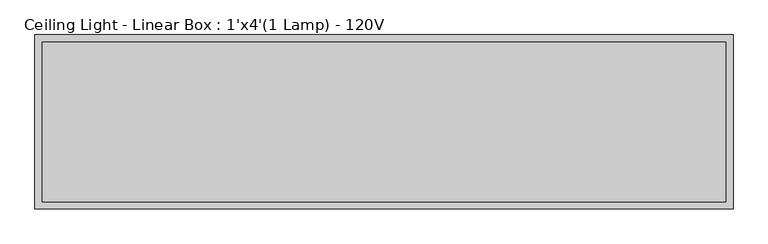
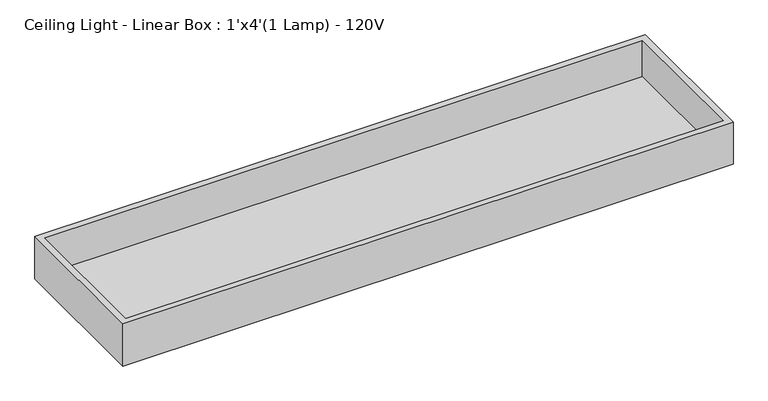
"""IFC4 building model written with IfcOpenShell, lengths in millimetres: light fixture geometry, Ceiling Light - Linear Box : 1'x4'(1 Lamp) - 120V."""

from ifc_helpers import new_model, si_unit, frame, origin, place, context, project, spatial, polyline, outline, extrude, source, transform, mapped, element, save


def ceiling_light_linear_box_1_x4_1_lamp_120v_8873ebfc(model_context):
    return source(origin(), model_context, "Body", "SweptSolid", [
        extrude(outline(polyline([(596.9, 139.7), (596.9, -139.7), (-596.9, -139.7), (-596.9, 139.7), (596.9, 139.7)])), frame((0.0, 0.0, 2355.85), z_axis=(0.0, 0.0, 1.0), x_axis=(1.0, 0.0, 0.0)), (0.0, 0.0, 1.0), 6.35),
        extrude(outline(polyline([(609.6, 152.4), (609.6, -152.4), (-609.6, -152.4), (-609.6, 152.4), (609.6, 152.4)]), holes=[polyline([(596.9, 139.7), (-596.9, 139.7), (-596.9, -139.7), (596.9, -139.7), (596.9, 139.7)])]), frame((0.0, 0.0, 2349.5), z_axis=(0.0, 0.0, 1.0), x_axis=(1.0, 0.0, 0.0)), (0.0, 0.0, 1.0), 88.9),
    ])


if __name__ == "__main__":
    model = new_model("IFC4")
    model_context = context("Model", 3, world=origin())
    ifc_project = project(units=[si_unit("LENGTHUNIT", "METRE", prefix="MILLI")], contexts=[model_context])
    site = spatial("IfcSite", under=ifc_project)
    building = spatial("IfcBuilding", under=site)
    placement = place(None, origin())
    ceiling_light_linear_box_1_x4_1_lamp_120v_shape = ceiling_light_linear_box_1_x4_1_lamp_120v_8873ebfc(model_context)
    element("IfcLightFixture", 1, ObjectType="Ceiling Light - Linear Box : 1'x4'(1 Lamp) - 120V", at=placement, inside=building, context=model_context, shape_type="MappedRepresentation", body=[
        mapped(ceiling_light_linear_box_1_x4_1_lamp_120v_shape, transform((0.0, 0.0, 0.0), x_axis=(1.0, 0.0, 0.0), y_axis=(0.0, 1.0, 0.0), z_axis=(0.0, 0.0, 1.0))),
    ])
    save(model, "model.ifc")

# Revit data of these elements
# Type "Ceiling Light - Linear Box : 1'x4'(1 Lamp) - 120V"
#   Assembly Code = "D5020210"
#   Lamp = "T-12"
#   Wattage = 40 W
#   built-in parameter 1150110 = 1 (stored number, unit not read)
#   built-in parameter 1114217 = 0.88 (stored number, unit not read)
#   built-in parameter 1150109 = 1 (stored number, unit not read)
#   built-in parameter 1150113 = 1 (stored number, unit not read)
#   built-in parameter 1150115 = 1 (stored number, unit not read)
#   built-in parameter 1150105 = 1002.68 (stored number, unit not read)
#   Light Source Symbol Size = 2' - 0"
#   built-in parameter 1150112 = 1 (stored number, unit not read)
#   built-in parameter 1150114 = 1 (stored number, unit not read)
#   built-in parameter 1150107 = 4230 (stored number, unit not read)
#   built-in parameter 1150106 = 10.0268 (stored number, unit not read)
#   Emit from Rectangle Width = 0' - 11"
#   Emit from Rectangle Length = 3' - 11"
#   built-in parameter 1150104 = 7.31611 (stored number, unit not read)
#   Ballast Voltage = 120 V
#   built-in parameter 1114218 = 0.88 (stored number, unit not read)
#   built-in parameter 1150133 = 10 (stored number, unit not read)
#   Box Length = 4' - 0"
#   Lumens = 3150 lm
#   Box Width = 1' - 0"
#   Apparent Load = 40 VA
#   built-in parameter 1150134 = 8
#   built-in parameter 1150137 = 1
#   Color Filter = 16777215
#   Ballast Number of Poles = 1
#   Diffuser Material = Glass, White, High Luminance
#   Light Box Material = Steel, Paint Finish, Ivory, Glossy
#   Emit Shape Visible in Rendering = no
#   Dimming Lamp Color Temperature Shift = (empty or 0)
#   Default Elevation = 0
# Element 1 (IfcLightFixture, "Ceiling Light - Linear Box : 1'x4'(1 Lamp) - 120V")
#   Materials on its faces: "Steel, Paint Finish, Ivory, Glossy", "Glass, White, High Luminance"
# Materials
#   "Glass, White, High Luminance": class "Glass", colour RGB 249 250 249, transparency 0.8, Description = "physical material", Cost = 0
#   "Steel, Paint Finish, Ivory, Glossy": class "Metal", colour RGB 247 247 239, transparency 0, Description = "Steel, paint finish, ivory, glossy", Cost = 0
